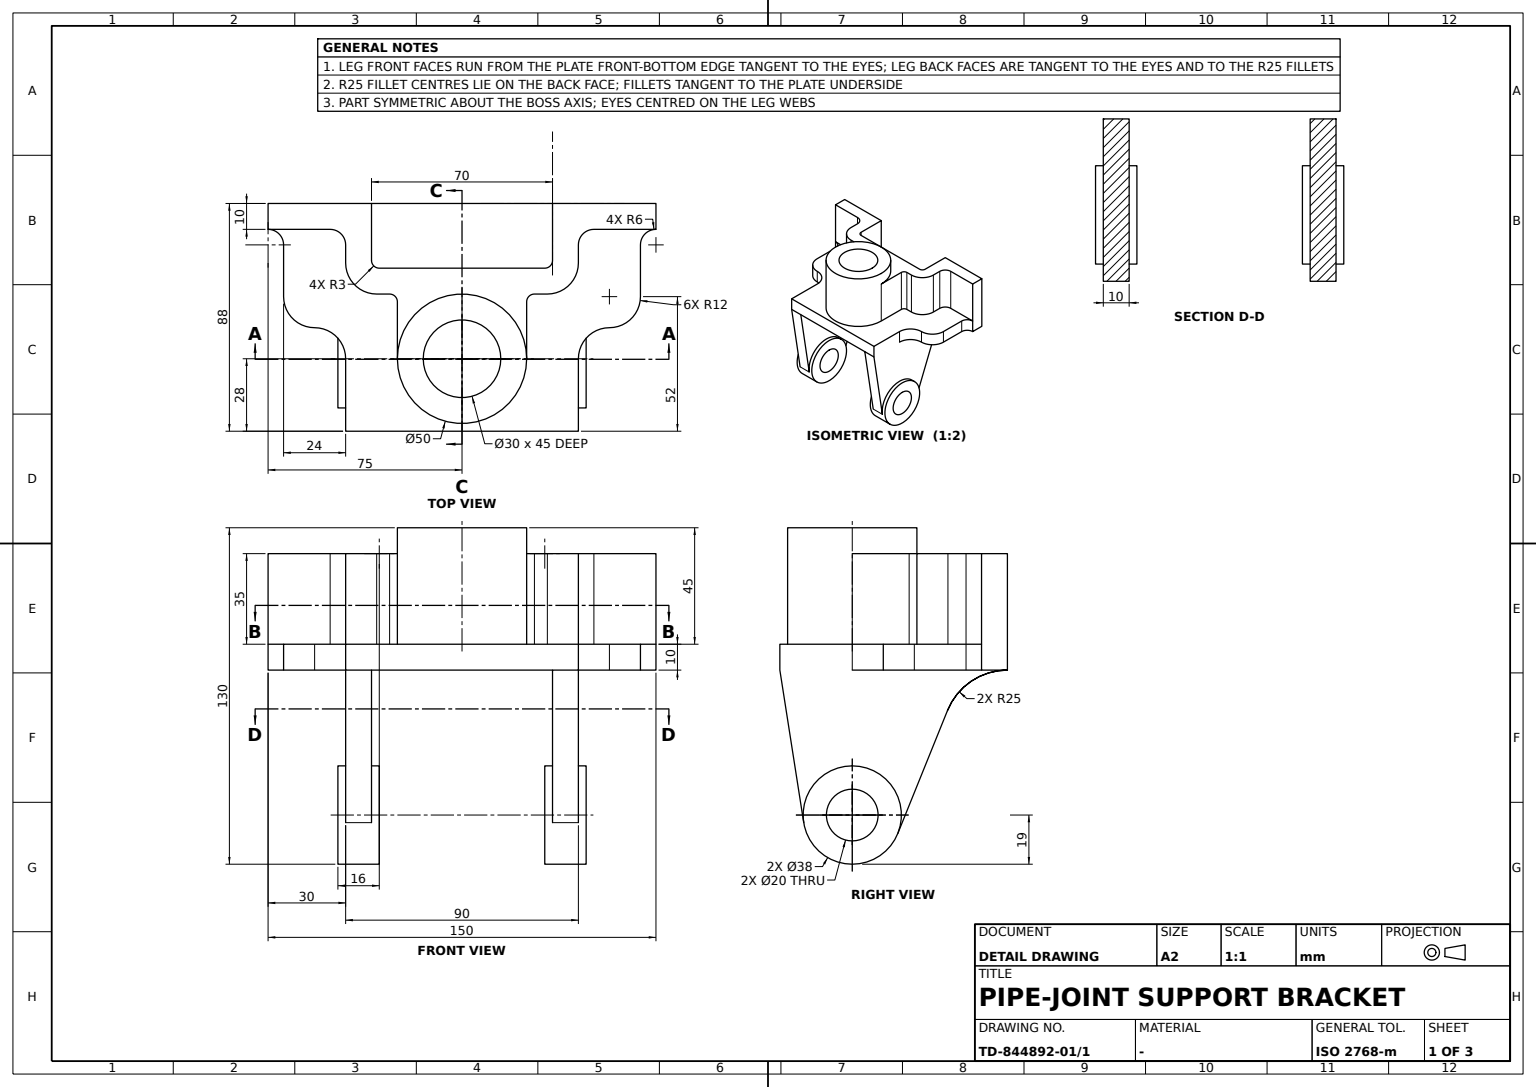
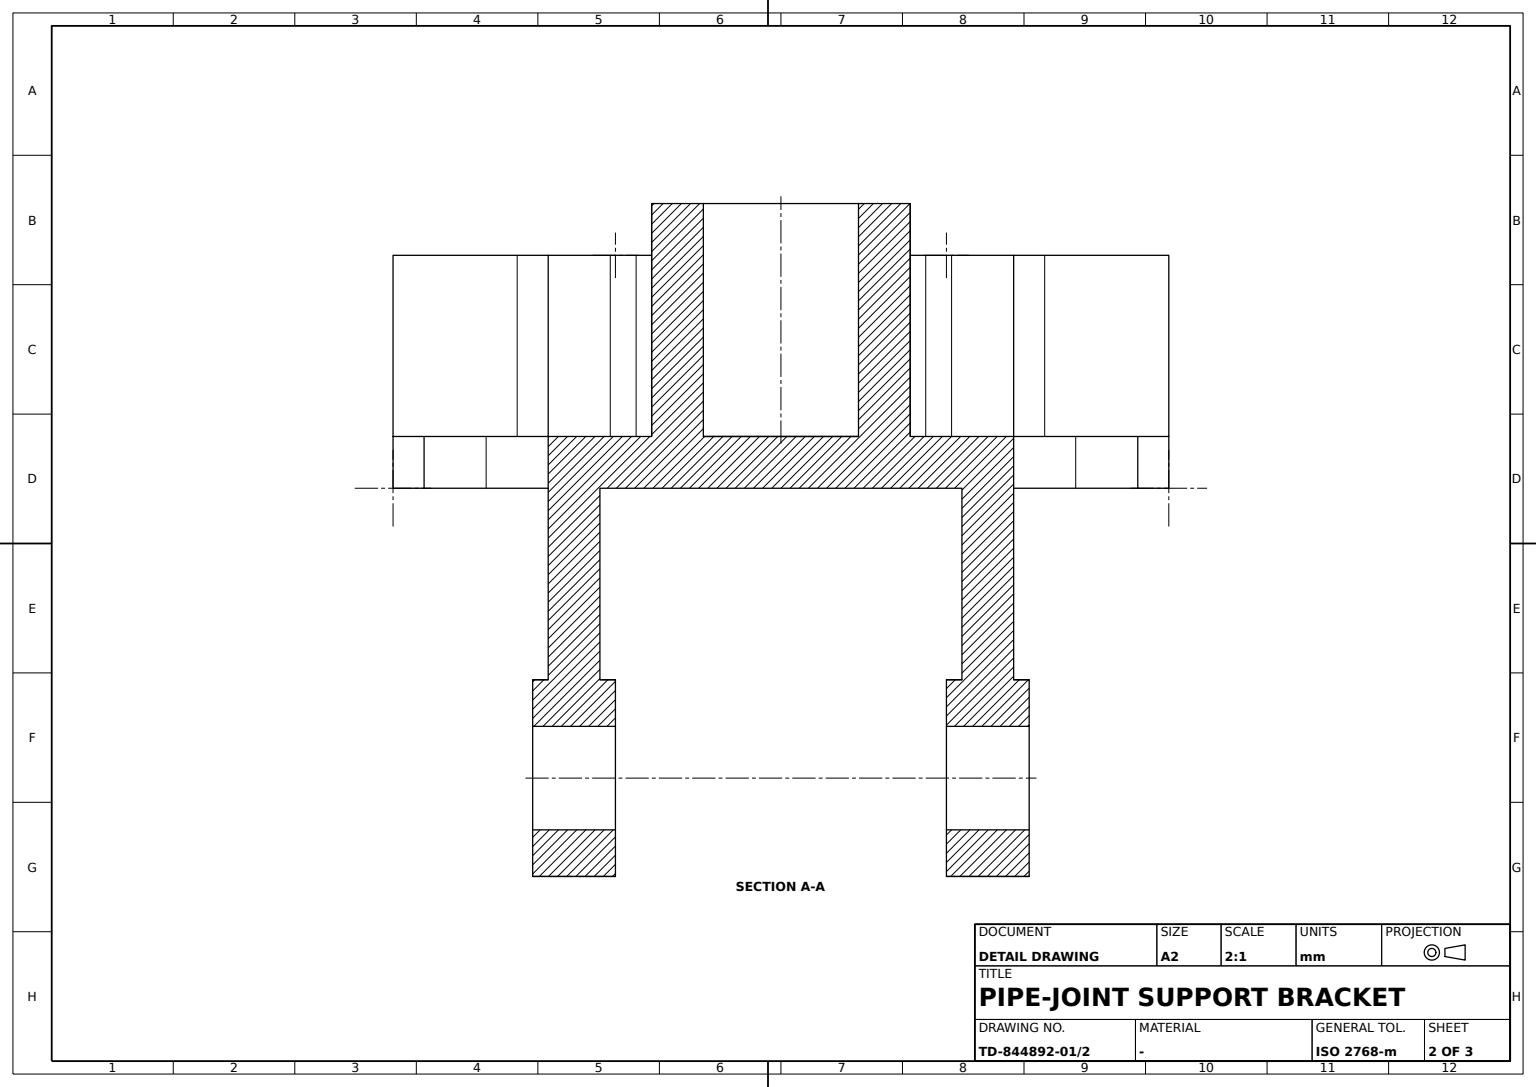
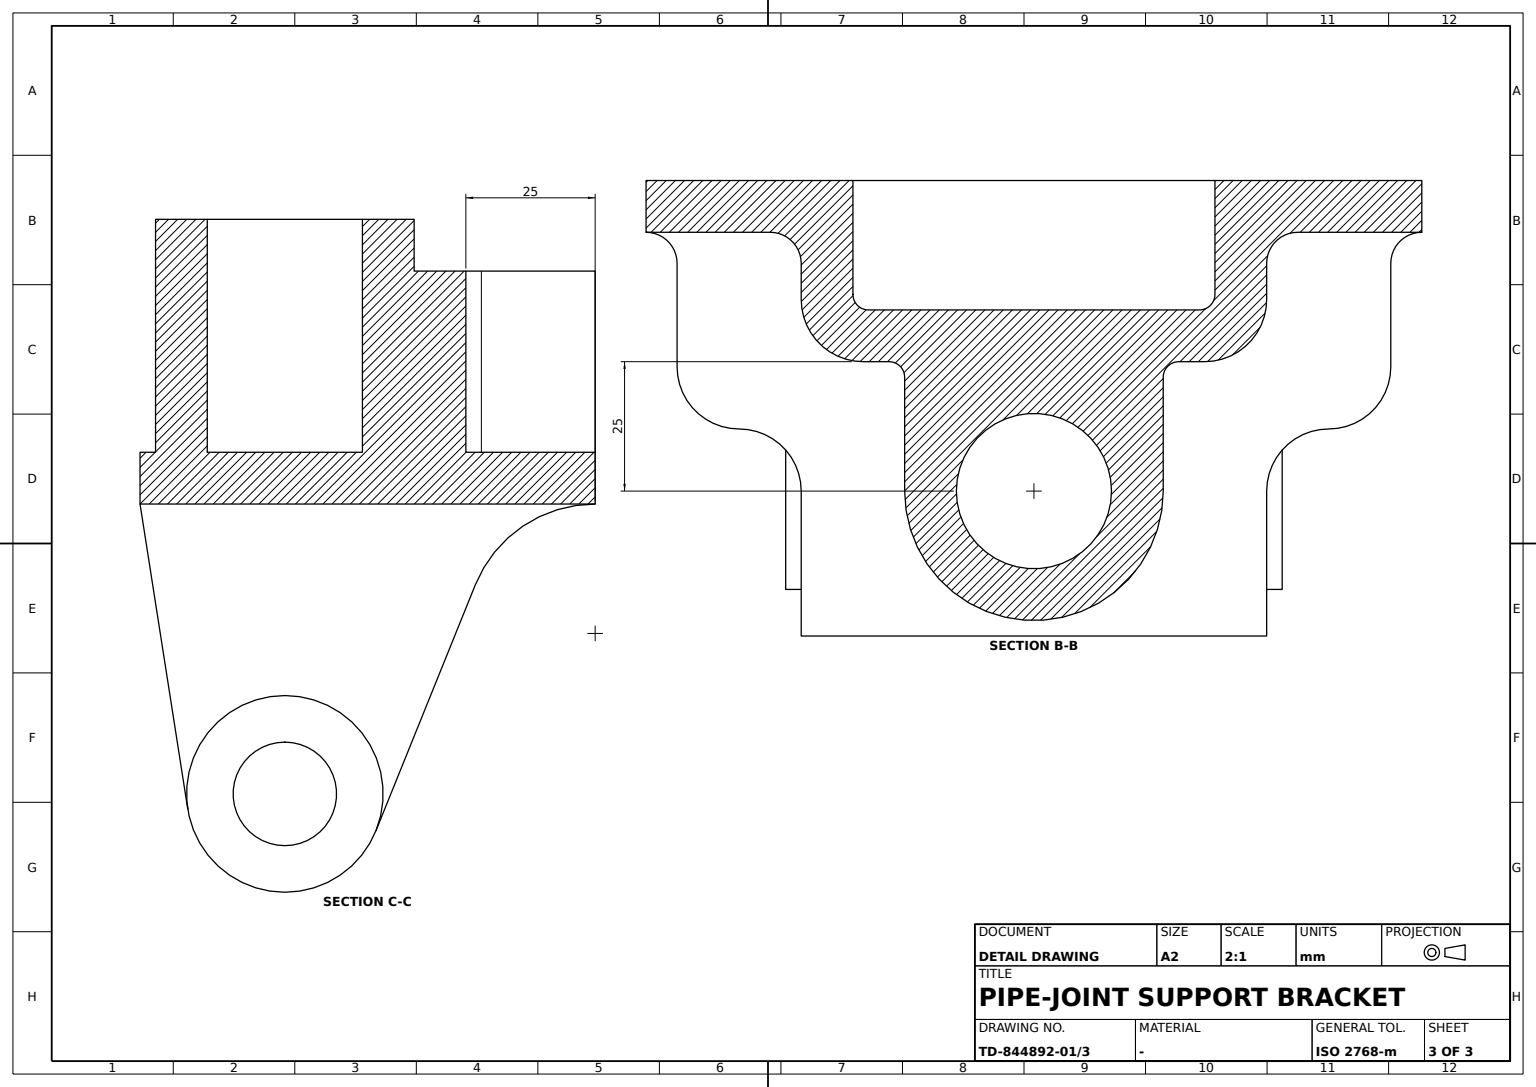
CATIA V5 part; units mm, degrees
sketch "Sketch1" plane through (0, 0, 0) normal (0, 0, 1) x (1, 0, 0)
  line L0 (-45, 0) -> (45, 0)
  point P0 (-45, 0)
  point P1 (45, 0)
  line L1 (45, 0) -> (45, 40)
  point P2 (45, 40)
  line L2 (45, 40) -> (69, 40)
  point P3 (69, 40)
  line L3 (69, 40) -> (69, 78)
  point P4 (69, 78)
  line L4 (69, 78) -> (75, 78)
  point P5 (75, 78)
  line L5 (75, 78) -> (75, 88)
  point P6 (75, 88)
  point P7 (-45, 0)
  point P8 (-45, 40)
  point P9 (-69, 40)
  point P10 (-69, 78)
  point P11 (-75, 78)
  point P12 (-75, 88)
  line L6 (-45, 0) -> (-45, 40)
  line L7 (-45, 40) -> (-69, 40)
  line L8 (-69, 40) -> (-69, 78)
  line L9 (-69, 78) -> (-75, 78)
  line L10 (-75, 78) -> (-75, 88)
  line L11 (-75, 88) -> (75, 88)
  dimension "length L0" = 90
  dimension "distance y axis P1" = 45
  dimension "length L1" = 40
  dimension "length L2" = 24
  dimension "length L3" = 38
  dimension "length L4" = 6
  dimension "length L5" = 10
  constraint coincidence P0 x-axis
  constraint horizontal L0 x-axis
  constraint horizontal L2 x-axis
  constraint horizontal L4 x-axis
  constraint horizontal L11 x-axis
  constraint vertical L1 y-axis
  constraint vertical L3 y-axis
  constraint vertical L5 y-axis
  constraint symmetry P1 P7 y-axis
  constraint symmetry P2 P8 y-axis
  constraint symmetry P3 P9 y-axis
  constraint symmetry P4 P10 y-axis
  constraint symmetry P5 P11 y-axis
  constraint symmetry P6 P12 y-axis
  constraint symmetry L1 L6 y-axis
  constraint symmetry L2 L7 y-axis
  constraint symmetry L3 L8 y-axis
  constraint symmetry L4 L9 y-axis
  constraint symmetry L5 L10 y-axis
extrude "Pad1" add sketch "Sketch1" along normal blind 10
fillet "Fillet1" radius 12 2 edges at (45, 40, 5) (-45, 40, 5)
fillet "Fillet2" radius 12 2 edges at (69, 40, 5) (-69, 40, 5)
fillet "Fillet3" radius 6 2 edges at (69, 78, 5) (-69, 78, 5)
sketch "Sketch2" plane through (0, 0, 10) normal (0, 0, 1) x (1, 0, 0)
  line L0 (75, 88) -> (-75, 88) construction
  point P0 (75, 88)
  point P1 (-75, 88)
  point P2 (75, 88)
  line L1 (-75, 88) -> (-75, 78)
  point P3 (-75, 78)
  line L2 (-75, 78) -> (-51, 78)
  point P4 (-45, 78)
  line L3 (-45, 72) -> (-45, 65)
  point P5 (-45, 53)
  point P6 (0, 28)
  point P7 (0, 45.5)
  line L4 (-35, 88) -> (-35, 66)
  point P8 (-35, 88)
  point P9 (-35, 63)
  line L5 (-25, 28) -> (-25, 50)
  point P10 (-25, 28)
  point P11 (-25, 53)
  line L6 (-33, 53) -> (-28, 53)
  point P12 (75, 88)
  point P13 (75, 78)
  point P14 (45, 78)
  point P15 (45, 53)
  point P16 (35, 88)
  point P17 (35, 63)
  point P18 (25, 28)
  point P19 (25, 53)
  line L7 (75, 78) -> (51, 78)
  line L8 (45, 72) -> (45, 65)
  line L9 (35, 88) -> (35, 66)
  line L10 (25, 28) -> (25, 50)
  line L11 (33, 53) -> (28, 53)
  line L12 (-32, 63) -> (32, 63)
  arc A0 (28, 53) -> (25, 50) centre (28, 50) ccw
  arc A1 (-28, 53) -> (-25, 50) centre (-28, 50) cw
  arc A2 (33, 53) -> (45, 65) centre (33, 65) ccw
  arc A3 (-33, 53) -> (-45, 65) centre (-33, 65) cw
  arc A4 (-35, 66) -> (-32, 63) centre (-32, 66) ccw
  arc A5 (32, 63) -> (35, 66) centre (32, 66) ccw
  arc A6 (-51, 78) -> (-45, 72) centre (-51, 72) cw
  arc A7 (51, 78) -> (45, 72) centre (51, 72) ccw
  arc A8 (25, 28) -> (-25, 28) centre (0, 28) ccw
  point P20 (0, 53)
  point P21 (-25, 28)
  line L13 (35, 88) -> (75, 88)
  line L14 (-75, 88) -> (-35, 88)
  line L15 (75, 88) -> (75, 78)
  dimension "distance L0 P5" = 35
  dimension "distance y axis P4" = 45
  dimension "distance L4 y axis" = 35
  dimension "distance P9 P5 y axis" = 10
  dimension "distance L0 P6" = 60
  dimension "distance P18 P19" = 25
  dimension "radius A0" = 3
  dimension "radius A1" = 3
  dimension "radius A2" = 12
  dimension "radius A3" = 12
  dimension "radius A4" = 3
  dimension "radius A5" = 3
  dimension "radius A6" = 6
  dimension "radius A7" = 6
  constraint horizontal L2 x-axis
  constraint horizontal L12 x-axis
  constraint horizontal L13 x-axis
  constraint horizontal L14 x-axis
  constraint vertical L3 y-axis
  constraint vertical L4 y-axis
  constraint vertical L15 y-axis
  constraint coincidence P6 y-axis
  constraint coincidence P7 y-axis
  constraint coincidence P8 L0
  constraint coincidence L11 P19
  constraint coincidence L10 P19
  constraint coincidence L6 P11
  constraint coincidence L5 P11
  constraint coincidence L11 P15
  constraint coincidence L8 P15
  constraint coincidence L6 P5
  constraint coincidence L3 P5
  constraint coincidence L4 P9
  constraint coincidence L12 P9
  constraint coincidence L12 P17
  constraint coincidence L9 P17
  constraint coincidence L2 P4
  constraint coincidence L3 P4
  constraint coincidence L7 P14
  constraint coincidence L8 P14
  constraint coincidence A8 P20
  constraint coincidence P20 y-axis
  constraint coincidence P0 P2
  constraint coincidence P10 P21
  constraint symmetry P1 P12 y-axis
  constraint symmetry P3 P13 y-axis
  constraint symmetry P4 P14 y-axis
  constraint symmetry P5 P15 y-axis
  constraint symmetry P8 P16 y-axis
  constraint symmetry P9 P17 y-axis
  constraint symmetry P10 P18 y-axis
  constraint symmetry P11 P19 y-axis
  constraint symmetry L2 L7 y-axis
  constraint symmetry L3 L8 y-axis
  constraint symmetry L4 L9 y-axis
  constraint symmetry L5 L10 y-axis
  constraint symmetry L6 L11 y-axis
  constraint tangency A0 L11
  constraint tangency A0 L10
  constraint tangency A1 L6
  constraint tangency A1 L5
  constraint tangency A2 L11
  constraint tangency A2 L8
  constraint tangency A3 L6
  constraint tangency A3 L3
  constraint tangency A4 L4
  constraint tangency A4 L12
  constraint tangency A5 L12
  constraint tangency A5 L9
  constraint tangency A6 L2
  constraint tangency A6 L3
  constraint tangency A7 L7
  constraint tangency A7 L8
  constraint tangency A8 L6
extrude "Pad2" add sketch "Sketch2" along normal blind 35
sketch "Sketch3" plane through (0, 0, 10) normal (0, 0, 1) x (1, 0, 0)
  circle A0 centre (0, 28) radius 25
  point P0 (0, 28)
  arc A1 (25, 28) -> (-25, 28) centre (0, 28) ccw construction
  arc A2 (25, 28) -> (-25, 28) centre (0, 28) ccw construction
  circle A3 centre (0, 28) radius 15
  dimension "radius A3" = 15
  constraint coincidence P0 y-axis
  constraint coincidence A0 A2
  constraint concentricity A0 A1
extrude "Pad3" add sketch "Sketch3" along normal blind 45
sketch "Sketch4" plane through (45, 0, 0) normal (1, 0, 0) x (0, 1, 0)
  arc A0 (45.614, -63.1238) -> (9.2287, -58.9392) centre (28, -56) ccw
  point P0 (28, -56)
  line L0 (0, 0) -> (9.2287, -58.9392)
  line L1 (45.614, -63.1238) -> (64.8237, -15.6266)
  point P1 (61, 0)
  line L2 (0, 0) -> (88, 0)
  point P2 (88, 0)
  arc A1 (88, 0) -> (64.8237, -15.6266) centre (88, -25) ccw
  point P3 (88, 0)
  dimension "distance y axis P0" = 28
  dimension "radius A0" = 19
  dimension "distance P1 y axis" = 61
  dimension "radius A1" = 25
  dimension "distance L2 P0" = 56
  constraint tangency L0 A0
  constraint tangency L1 A0
  constraint tangency A1 L1
  constraint tangency A1 L2
  constraint coincidence P1 x-axis
  constraint coincidence P2 P3
  constraint horizontal L2 x-axis
extrude "Pad4" add sketch "Sketch4" against normal blind 10
ref_plane "Plane1" through (40, 0, 0) normal (1, 0, 0) x (0, -1, 0)
sketch "Sketch5" plane through (40, 0, 0) normal (-1, 0, 0) x (0, -1, 0)
  circle A0 centre (-28, -56) radius 19
  point P0 (-28, -56)
  arc A1 (-9.2287, -58.9392) -> (-45.614, -63.1238) centre (-28, -56) ccw construction
  circle A2 centre (-28, -56) radius 10
  point P1 (-28, -56)
  dimension "radius A2" = 10
  constraint coincidence A0 A1
  constraint coincidence P1 P0
extrude "Pad5" add sketch "Sketch5" along normal mid plane 16
mirror "Mirror1" about plane through (0, 0, 0) normal (1, 0, 0) of "Pad4", "Pad5"
